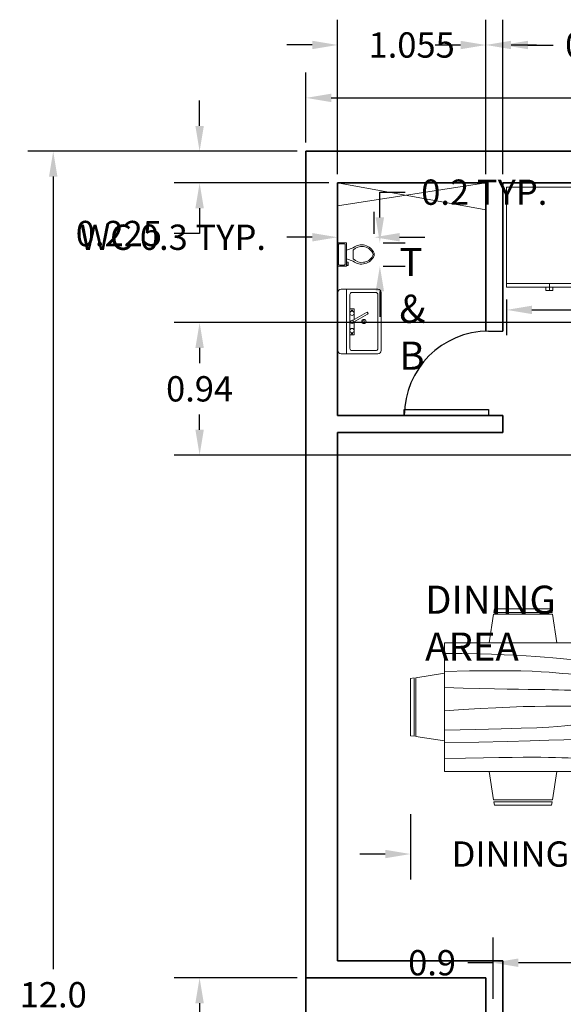
# Model space of a CAD drawing. Units: metres. Extents: x 4.8 to 18.3, y 28.2 to 89.8.
# Tile 2 of 4: x 4.8 to 8.6, y 36.6 to 43.6. Entities that reach past the tile are written whole.
import ezdxf

# ---------------------------------------------------------------- set-up
doc = ezdxf.new("R2010")
doc.units = ezdxf.units.M
doc.header["$MEASUREMENT"] = 0
doc.layers.get('Defpoints').update_dxf_attribs({"color": 3})
for name, color, linetype, lineweight in [('A-ANNO-DIMS', 2, 'Continuous', 18), ('A-AREA-IDEN', 7, 'Continuous', 25), ('A-DOOR', 3, 'Continuous', 25), ('A-EQPM', 8, 'Continuous', 18), ('A-FLOR-FIXT', 9, 'Continuous', 18), ('A-FURN', 8, 'Continuous', 18), ('A-WALL', 7, 'Continuous', 35)]:
    doc.layers.add(name, color=color, linetype=linetype, lineweight=lineweight)
doc.styles.get("Standard").update_dxf_attribs({"font": 'arial.ttf'})
doc.dimstyles.get("Standard").update_dxf_attribs({"dimtxt": 0.18, "dimasz": 0.18, "dimexe": 0.18, "dimexo": 0.0625, "dimgap": 0.09, "dimtad": 0, "dimtih": 1, "dimtoh": 1, "dimdec": 1, "dimzin": 0, "dimdsep": 46, "dimtxsty": 'Standard', "dimcen": 0.09, "dimadec": 0, "dimazin": 0, "dimtfac": 1, "dimtdec": 1, "dimtofl": 0, "dimtmove": 0, "dimatfit": 3, "dimfxl": 1, "dimtolj": 1, "dimtzin": 0, "dimarcsym": 0})

# ---------------------------------------------------------------- blocks, each defined once
blk = doc.blocks.new('*U3')
for p, q in [((0, 0), (0, -100)), ((600, 0), (600, -100))]:
    blk.add_line(p, q)
blk.add_lwpolyline([(0, 0), (0, 600), (43.75, 600), (43.75, 0)], close=True)
blk.add_arc((0, 0), 600, 0, 90)
blk = doc.blocks.new('Toilet - top')
for p, q in [((-10, -8.5), (-8, -8.5)), ((-10, -9.5), (-10, -8.5)), ((-8, -8.5), (-8, -8)), ((-7, -8), (-7, -9.5)), ((-4, -8), (-6, -14)), ((4, -8), (6, -14)), ((9.5, -6), (9.5, -2)), ((-7, -9.5), (-10, -9.5)), ((4, -14), (-4, -14))]:
    blk.add_line(p, q)
blk.add_lwpolyline([(10.5, -8), (10.5, 0), (-10.5, 0), (-10.5, -8)], close=True)
for points in [[(-9.5, -2), (-9.5, -6)], [(8.5, -1), (-8.5, -1)], [(-8.5, -7), (8.5, -7)]]:
    blk.add_lwpolyline(points)
for centre, radius, start, end in [((-8.62, -1.88), 0.884, 81.8699, 188.1301), ((-8.62, -6.12), 0.884, 171.8699, 278.1301), ((8.62, -1.88), 0.884, 351.8699, 98.1301), ((8.62, -6.12), 0.884, 261.8699, 8.1301), ((3.52, -21.58), 12.17, 141.46911, 247.97143), ((4.2, -21.82), 11.33, 136.36773, 238.94682), ((-3.52, -21.58), 12.17, 292.02843, 38.53071), ((-4.2, -21.82), 11.33, 301.05301, 43.63209), ((0, -27.88), 4, 245.73182, 294.26817), ((0, -29), 4, 254.86053, 285.13947)]:
    blk.add_arc(centre, radius, start, end)
blk = doc.blocks.new('Sink-single - 30 in top')
blk.add_line((-15, -3.999996), (15, -3.999996))
for points in [[(-13.5, 0), (13.5, 0)], [(-15, -18.499996), (-15, -1.5)], [(15, -1.5), (15, -18.499996)], [(-13.5, -17.499996), (-13.5, -6.499996)], [(-12.5, -5.499996), (12.5, -5.499996)], [(13.5, -6.499996), (13.5, -17.499996)], [(13.5, -19.999996), (-13.5, -19.999996)], [(12.5, -18.499996), (-12.5, -18.499996)]]:
    blk.add_lwpolyline(points)
for radius in [1, 0.5]:
    blk.add_circle((0, -11.999996), radius)
for centre, radius, start, end in [((-13.5, -1.5), 1.5, 90, 180), ((13.5, -1.5), 1.5, 0, 90), ((-12.5, -6.499996), 1, 90, 180), ((12.5, -6.499996), 1, 0, 90), ((-12.5, -17.499996), 1, 180, 270), ((12.5, -17.499996), 1, 270, 0), ((-13.5, -18.499996), 1.5, 180, 270), ((13.5, -18.499996), 1.5, 270, 0)]:
    blk.add_arc(centre, radius, start, end)
blk = doc.blocks.new('Faucet - kit sink top')
for p, q in [((-5.5, -0.75), (-5.5, -1.25)), ((-4.94278, -0.75), (-5.5, -0.75)), ((-5.5, -1.25), (-4.94278, -1.25)), ((-0.14775, -1.7441), (3.56698, -8.1782)), ((4.43301, -7.6782), (0.71828, -1.2441)), ((4.94278, -0.75), (5.5, -0.75)), ((5.5, -1.25), (4.94278, -1.25)), ((5.5, -0.75), (5.5, -1.25))]:
    blk.add_line(p, q)
blk.add_lwpolyline([(-0.00587, -2), (-6, -2), (-6, 0), (6, 0), (6, -2), (1.15195, -2)])
for centre, radius in [((-4, -1), 1), ((4, -1), 1), ((0, -1), 0.75)]:
    blk.add_circle(centre, radius)
blk.add_arc((4, -7.9282), 0.5, 210, 30)
blk = doc.blocks.new('Refrigerator-2 door - 36 in top')
for p, q in [((0, -26.999999), (36, -26.999999)), ((12, -26.999999), (12, -28.999999)), ((11, -27.999999), (11, -28.999999)), ((11, -28.999999), (13, -28.999999)), ((13, -28.999999), (13, -27.999999))]:
    blk.add_line(p, q)
blk.add_lwpolyline([(0, -27.999999), (0, 0), (36, 0), (36, -27.999999)], close=True)
blk = doc.blocks.new('Dining Set - 36 x 72 in.')
for p, q in [((-22.2343, 26.00059), (-23.4847, 17.99762)), ((-22.2304, 26), (-5.7608, 26)), ((-22, 27.5), (-22.1562, 26.50042)), ((-5.8416, 26.5), (-22.1534, 26.5)), ((-22, 27.5), (-6, 27.5)), ((-5.8437, 26.49966), (-6, 27.5)), ((-4.5152, 17.99762), (-5.7655, 25.99926)), ((5.7657, 26.00059), (4.5153, 17.99762)), ((5.7696, 26), (22.2392, 26)), ((6, 27.5), (5.8438, 26.50042)), ((22.1584, 26.5), (5.8466, 26.5)), ((6, 27.5), (22, 27.5)), ((22.1563, 26.49966), (22, 27.5)), ((23.4848, 17.99762), (22.2345, 25.99926)), ((36, 18), (-36, 18)), ((-36, 18), (-36, -18)), ((36, -18), (36, 18)), ((-44.0006, 8.23428), (-35.9976, 9.48474)), ((44.0006, 8.23428), (35.9976, 9.48474)), ((-45.5, 8), (-44.5004, 8.15617)), ((-45.5, 8), (-45.5, -8)), ((-44.5, -8.15843), (-44.5, 8.15338)), ((-44, 8.23041), (-44, -8.23915)), ((44, 8.23041), (44, -8.23915)), ((44.5, -8.15843), (44.5, 8.15338)), ((45.5, 8), (44.5005, 8.15617)), ((45.5, 8), (45.5, -8)), ((-44.4997, -8.15631), (-45.5, -8)), ((-35.9976, -9.48476), (-43.9993, -8.2345)), ((35.9976, -9.48476), (43.9993, -8.2345)), ((44.4997, -8.15631), (45.5, -8)), ((-36, -18), (36, -18)), ((-22.2343, -26.0006), (-23.4847, -17.99762)), ((-4.5152, -17.99762), (-5.7655, -25.99928)), ((5.7657, -26.0006), (4.5153, -17.99762)), ((23.4848, -17.99762), (22.2345, -25.99928)), ((-22.2304, -26), (-5.7608, -26)), ((-22, -27.5), (-22.1562, -26.50044)), ((-5.8416, -26.5), (-22.1534, -26.5)), ((-22, -27.5), (-6, -27.5)), ((-5.8437, -26.49967), (-6, -27.5)), ((5.7696, -26), (22.2392, -26)), ((6, -27.5), (5.8438, -26.50044)), ((22.1584, -26.5), (5.8466, -26.5)), ((6, -27.5), (22, -27.5)), ((22.1563, -26.49967), (22, -27.5))]:
    blk.add_line(p, q)
for points in [[(-36, 15), (-31.1772, 14.97754), (-26.8079, 14.91406), (-22.8538, 14.81543), (-19.276, 14.6875), (-16.0362, 14.53613), (-13.0957, 14.36718), (-10.4159, 14.18652), (-7.9583, 14), (-5.6904, 13.81315), (-3.6035, 13.63021), (-1.6954, 13.45508), (0.0365, 13.29166), (1.5945, 13.14388), (2.9811, 13.01562), (4.1988, 12.9108), (5.25, 12.83333), (6.1393, 12.78613), (6.8802, 12.76823), (7.4883, 12.77767), (7.9792, 12.8125), (8.3685, 12.87077), (8.6719, 12.95052), (8.9049, 13.0498), (9.0833, 13.16666), (9.2205, 13.29899), (9.3216, 13.44401), (9.3895, 13.59879), (9.4271, 13.76041), (9.4373, 13.92594), (9.4232, 14.09245), (9.3875, 14.257), (9.3333, 14.41666), (9.2638, 14.56917), (9.1836, 14.71484), (9.0975, 14.85465), (9.0104, 14.98958), (8.9272, 15.1206), (8.8529, 15.2487), (8.7922, 15.37483), (8.75, 15.5), (8.7305, 15.62467), (8.7344, 15.74739), (8.7617, 15.86621), (8.8125, 15.97916), (8.8867, 16.08431), (8.9844, 16.17968), (9.1055, 16.26334), (9.25, 16.33333), (9.4189, 16.38802), (9.6172, 16.42708), (9.8506, 16.45052), (10.125, 16.45833), (10.4463, 16.45052), (10.8203, 16.42708), (11.2529, 16.38802), (11.75, 16.33333), (12.3184, 16.26318), (12.9694, 16.17838), (13.7151, 16.07991), (14.5677, 15.96875), (15.5395, 15.84586), (16.6426, 15.71224), (17.8893, 15.56884), (19.2917, 15.41666), (20.859, 15.25667), (22.5879, 15.08984), (24.4721, 14.91715), (26.5052, 14.73958), (28.6809, 14.5581), (30.9929, 14.3737), (33.4347, 14.18733), (36, 14)], [(-36, 10), (-28.9766, 10.14274), (-23.1725, 10.20442), (-18.4241, 10.19775), (-14.5677, 10.13541), (-11.4399, 10.03011), (-8.877, 9.89453), (-6.7154, 9.74137), (-4.7917, 9.58333), (-2.9698, 9.43082), (-1.2246, 9.28515), (0.4415, 9.14534), (2.026, 9.01041), (3.5266, 8.87939), (4.9408, 8.7513), (6.266, 8.62516), (7.5, 8.5), (8.6411, 8.37549), (9.6914, 8.2539), (10.6538, 8.13818), (11.5312, 8.03125), (12.3267, 7.93603), (13.043, 7.85547), (13.6831, 7.79248), (14.25, 7.75), (14.7471, 7.7303), (15.1797, 7.73307), (15.5537, 7.75732), (15.875, 7.80208), (16.1494, 7.86637), (16.3828, 7.94922), (16.5811, 8.04964), (16.75, 8.16666), (16.8944, 8.29915), (17.0143, 8.44531), (17.1089, 8.60319), (17.1771, 8.77083), (17.218, 8.94629), (17.2305, 9.1276), (17.2137, 9.31282), (17.1667, 9.5), (17.0895, 9.6875), (16.987, 9.875), (16.8649, 10.0625), (16.7292, 10.25), (16.5856, 10.4375), (16.4401, 10.625), (16.2985, 10.8125), (16.1667, 11), (16.05, 11.18733), (15.9518, 11.3737), (15.8752, 11.5581), (15.8229, 11.73958), (15.798, 11.91715), (15.8034, 12.08984), (15.842, 12.25667), (15.9167, 12.41666), (16.0295, 12.56836), (16.1784, 12.70833), (16.3605, 12.83268), (16.5729, 12.9375), (16.8127, 13.01888), (17.0768, 13.07291), (17.3625, 13.0957), (17.6667, 13.08333), (17.9894, 13.03312), (18.3418, 12.94726), (18.7382, 12.82918), (19.1927, 12.68229), (19.7195, 12.51001), (20.3327, 12.31575), (21.0465, 12.10294), (21.875, 11.875), (22.8357, 11.63354), (23.959, 11.37304), (25.2786, 11.08618), (26.8282, 10.76562), (28.6414, 10.40405), (30.752, 9.99414), (33.1936, 9.52856), (36, 9)], [(-36, 5.5), (-30.7157, 5.3348), (-26.069, 5.20963), (-21.9946, 5.11767), (-18.4271, 5.05208), (-15.3009, 5.00602), (-12.5508, 4.97265), (-10.1112, 4.94515), (-7.9167, 4.91666), (-5.909, 4.88167), (-4.0586, 4.83984), (-2.3429, 4.79215), (-0.7396, 4.73958), (0.7739, 4.6831), (2.22, 4.6237), (3.6213, 4.56233), (5, 4.5), (6.373, 4.43782), (7.7344, 4.3776), (9.0723, 4.32129), (10.375, 4.27083), (11.6309, 4.22819), (12.8281, 4.19531), (13.9551, 4.17415), (15, 4.16666), (15.954, 4.17448), (16.819, 4.19791), (17.6001, 4.23698), (18.3021, 4.29166), (18.9299, 4.36198), (19.4883, 4.44791), (19.9823, 4.54948), (20.4167, 4.66666), (20.7969, 4.79899), (21.1302, 4.94401), (21.4245, 5.09879), (21.6875, 5.26041), (21.9271, 5.42594), (22.1511, 5.59245), (22.3672, 5.757), (22.5834, 5.91666), (22.8065, 6.06868), (23.0404, 6.21093), (23.2879, 6.34147), (23.5521, 6.45833), (23.8358, 6.55957), (24.142, 6.64323), (24.4735, 6.70735), (24.8334, 6.75), (25.2235, 6.76969), (25.642, 6.76692), (26.0858, 6.74267), (26.5521, 6.69791), (27.0379, 6.63362), (27.5404, 6.55078), (28.0565, 6.45036), (28.5834, 6.33333), (29.1242, 6.19987), (29.7071, 6.04687), (30.3661, 5.87044), (31.1354, 5.66666), (32.0493, 5.43164), (33.142, 5.16146), (34.4475, 4.85221), (36, 4.5)], [(-36, -1), (-30.7915, -0.6591), (-26.0195, -0.38216), (-21.6519, -0.16284), (-17.6563, 0.00521), (-14.0005, 0.12833), (-10.6523, 0.21289), (-7.5796, 0.26522), (-4.75, 0.29166), (-2.134, 0.29793), (0.2878, 0.28711), (2.5317, 0.26163), (4.6146, 0.22396), (6.5529, 0.17651), (8.3633, 0.12174), (10.0623, 0.06209), (11.6667, 0), (13.1899, -0.06201), (14.6341, -0.1211), (15.9982, -0.17432), (17.2813, -0.21875), (18.4823, -0.25147), (19.6003, -0.26953), (20.6343, -0.27002), (21.5834, -0.25), (22.4481, -0.20768), (23.2357, -0.14584), (23.9549, -0.06836), (24.6146, 0.02083), (25.2235, 0.11784), (25.7904, 0.21875), (26.3241, 0.31966), (26.8334, 0.41666), (27.3265, 0.50618), (27.8099, 0.58593), (28.2894, 0.65397), (28.7709, 0.70833), (29.2601, 0.74707), (29.763, 0.76823), (30.2855, 0.76985), (30.8334, 0.75), (31.4088, 0.70784), (31.9994, 0.64713), (32.589, 0.57275), (33.1615, 0.48958), (33.7008, 0.4025), (34.1908, 0.3164), (34.6153, 0.23616), (34.9584, 0.16666), (35.2099, 0.11165), (35.3848, 0.07031), (35.504, 0.04069), (35.5886, 0.02083), (35.6594, 0.00879), (35.7377, 0.0026), (35.8442, 0.00032), (36, 0)], [(-36, -6.5), (-27.1843, -6.31267), (-20.084, -6.1263), (-14.469, -5.9419), (-10.1094, -5.76042), (-6.7752, -5.58285), (-4.2363, -5.41016), (-2.2629, -5.24333), (-0.625, -5.08334), (0.8708, -4.93099), (2.2715, -4.78646), (3.5872, -4.64974), (4.8281, -4.52084), (6.0046, -4.39974), (7.127, -4.28646), (8.2053, -4.18099), (9.25, -4.08334), (10.2705, -3.99382), (11.2734, -3.91407), (12.2647, -3.84603), (13.25, -3.79167), (14.2354, -3.75293), (15.2266, -3.73177), (16.2295, -3.73015), (17.25, -3.75), (18.2912, -3.79248), (19.3451, -3.85547), (20.4009, -3.93604), (21.4479, -4.03125), (22.4754, -4.13819), (23.4727, -4.25391), (24.4289, -4.37549), (25.3334, -4.5), (26.1785, -4.62492), (26.9694, -4.74935), (27.7145, -4.87281), (28.4219, -4.99479), (29.1, -5.11483), (29.7572, -5.23242), (30.4016, -5.34709), (31.0417, -5.45834), (31.6837, -5.56437), (32.3262, -5.65821), (32.9658, -5.73153), (33.599, -5.77604), (34.2224, -5.78345), (34.8327, -5.74545), (35.4264, -5.65373), (36, -5.5)], [(-36, -10), (-26.4022, -9.81299), (-18.4675, -9.62891), (-11.9839, -9.45069), (-6.7396, -9.28125), (-2.5226, -9.12354), (0.8789, -8.98047), (3.6769, -8.85498), (6.0833, -8.75), (8.2767, -8.66765), (10.3021, -8.60677), (12.1712, -8.56543), (13.8958, -8.54167), (15.4876, -8.53353), (16.9583, -8.53907), (18.3197, -8.55632), (19.5834, -8.58334), (20.7616, -8.61841), (21.8685, -8.66081), (22.9188, -8.71004), (23.9271, -8.76563), (24.9081, -8.82707), (25.8763, -8.89388), (26.8465, -8.96558), (27.8334, -9.04167), (28.8474, -9.12118), (29.8828, -9.20117), (30.93, -9.27824), (31.9792, -9.34896), (33.0205, -9.40991), (34.0443, -9.45768), (35.0407, -9.48885), (36, -9.5)], [(-36, -14.5), (-30.0881, -14.33513), (-25.0332, -14.21224), (-20.7312, -14.12647), (-17.0781, -14.07292), (-13.97, -14.04671), (-11.3027, -14.04297), (-8.9724, -14.05681), (-6.875, -14.08334), (-4.9224, -14.11833), (-3.0905, -14.16016), (-1.3709, -14.20785), (0.2448, -14.26042), (1.7647, -14.3169), (3.1973, -14.3763), (4.5507, -14.43767), (5.8333, -14.5), (7.0554, -14.5621), (8.235, -14.62175), (9.3922, -14.67652), (10.5469, -14.72396), (11.7192, -14.76164), (12.929, -14.78711), (14.1965, -14.79794), (15.5417, -14.79167), (16.9933, -14.76424), (18.6152, -14.70508), (20.4804, -14.60197), (22.6615, -14.44271), (25.2312, -14.21509), (28.2624, -13.9069), (31.8277, -13.50594), (36, -13)]]:
    blk.add_lwpolyline(points)
blk = doc.blocks.new('*D18')
at = {"layer": 'A-ANNO-DIMS', "color": 0, "lineweight": -2, "transparency": 16777216}
for p, q in [((6.731, 42.6633), (4.8163, 42.6633)), ((4.9963, 42.4833), (4.9963, 36.8452)), ((4.9963, 30.8433), (4.9963, 36.4813)), ((6.731, 30.6633), (4.8163, 30.6633))]:
    blk.add_line(p, q, dxfattribs=at)
at = {"layer": 'A-ANNO-DIMS', "color": 0, "transparency": 16777216}
for points in [[(4.9663, 42.4833), (5.0263, 42.4833), (4.9963, 42.6633)], [(4.9663, 30.8433), (5.0263, 30.8433), (4.9963, 30.6633)]]:
    blk.add_solid(points, dxfattribs=at)
at = {"layer": 'Defpoints', "color": 0, "transparency": 16777216}
for p in [(6.7935, 42.6633), (4.9963, 30.6633), (6.7935, 30.6633)]:
    blk.add_point(p, dxfattribs=at)
at = {"layer": 'A-ANNO-DIMS', "color": 0, "transparency": 16777216, "insert": (4.9963, 36.6633), "char_height": 0.18, "attachment_point": 5}
blk.add_mtext('\\A1;12.0', dxfattribs=at)
blk = doc.blocks.new('*D22')
at = {"layer": 'A-ANNO-DIMS', "color": 0, "lineweight": -2, "transparency": 16777216}
for p, q in [((6.7935, 42.7258), (6.7935, 43.223)), ((12.2935, 42.7258), (12.2935, 43.223)), ((6.9735, 43.043), (9.289, 43.043)), ((12.1135, 43.043), (9.798, 43.043))]:
    blk.add_line(p, q, dxfattribs=at)
at = {"layer": 'A-ANNO-DIMS', "color": 0, "transparency": 16777216}
for points in [[(6.9735, 43.073), (6.9735, 43.013), (6.7935, 43.043)], [(12.1135, 43.073), (12.1135, 43.013), (12.2935, 43.043)]]:
    blk.add_solid(points, dxfattribs=at)
at = {"layer": 'Defpoints', "color": 0, "transparency": 16777216}
for p in [(12.2935, 43.043), (6.7935, 42.6633), (12.2935, 42.6633)]:
    blk.add_point(p, dxfattribs=at)
at = {"layer": 'A-ANNO-DIMS', "color": 0, "transparency": 16777216, "insert": (9.5435, 43.043), "char_height": 0.18, "attachment_point": 5}
blk.add_mtext('\\A1;5.5', dxfattribs=at)
blk = doc.blocks.new('*D32')
at = {"layer": 'A-ANNO-DIMS', "color": 0, "lineweight": -2, "transparency": 16777216}
for p, q in [((7.0185, 42.0749), (7.0185, 42.2317)), ((7.2803, 42.0749), (7.2803, 42.2317)), ((6.8385, 42.0517), (6.6585, 42.0517)), ((7.4603, 42.0517), (7.6403, 42.0517))]:
    blk.add_line(p, q, dxfattribs=at)
at = {"layer": 'A-ANNO-DIMS', "color": 0, "transparency": 16777216}
for points in [[(6.8385, 42.0817), (6.8385, 42.0217), (7.0185, 42.0517)], [(7.4603, 42.0817), (7.4603, 42.0217), (7.2803, 42.0517)]]:
    blk.add_solid(points, dxfattribs=at)
at = {"layer": 'Defpoints', "color": 0, "transparency": 16777216}
for p in [(7.0185, 42.0517), (7.0185, 42.0124), (7.2803, 42.0124)]:
    blk.add_point(p, dxfattribs=at)
at = {"layer": 'A-ANNO-DIMS', "color": 0, "transparency": 16777216, "insert": (5.8474, 42.0517), "char_height": 0.18, "attachment_point": 5}
blk.add_mtext('\\A1;WC 0.3 TYP.', dxfattribs=at)
blk = doc.blocks.new('*D33')
at = {"layer": 'A-ANNO-DIMS', "color": 0, "lineweight": -2, "transparency": 16777216}
for p, q in [((7.3196, 42.1924), (7.3196, 42.3724)), ((7.3196, 42.3724), (7.4996, 42.3724)), ((7.3428, 42.0124), (7.4996, 42.0124)), ((7.3428, 41.846), (7.4996, 41.846)), ((7.3196, 41.666), (7.3196, 41.486))]:
    blk.add_line(p, q, dxfattribs=at)
at = {"layer": 'A-ANNO-DIMS', "color": 0, "transparency": 16777216}
for points in [[(7.2896, 42.1924), (7.3496, 42.1924), (7.3196, 42.0124)], [(7.2896, 41.666), (7.3496, 41.666), (7.3196, 41.846)]]:
    blk.add_solid(points, dxfattribs=at)
at = {"layer": 'Defpoints', "color": 0, "transparency": 16777216}
for p in [(7.2803, 42.0124), (7.3196, 42.0124), (7.2803, 41.846)]:
    blk.add_point(p, dxfattribs=at)
at = {"layer": 'A-ANNO-DIMS', "color": 0, "transparency": 16777216, "insert": (8.0626, 42.3724), "char_height": 0.18, "attachment_point": 5}
blk.add_mtext('\\A1;0.2 TYP.', dxfattribs=at)
blk = doc.blocks.new('*D36')
at = {"layer": 'A-ANNO-DIMS', "color": 0, "lineweight": -2, "transparency": 16777216}
for p, q in [((8.2211, 41.6097), (8.2211, 41.355)), ((9.1355, 41.6097), (9.1355, 41.355)), ((8.4011, 41.535), (8.9555, 41.535)), ((9.1355, 41.535), (9.3155, 41.535))]:
    blk.add_line(p, q, dxfattribs=at)
at = {"layer": 'A-ANNO-DIMS', "color": 0, "transparency": 16777216}
for points in [[(8.4011, 41.565), (8.4011, 41.505), (8.2211, 41.535)], [(8.9555, 41.565), (8.9555, 41.505), (9.1355, 41.535)]]:
    blk.add_solid(points, dxfattribs=at)
at = {"layer": 'Defpoints', "color": 0, "transparency": 16777216}
for p in [(8.2211, 41.6722), (9.1355, 41.6722), (9.1355, 41.535)]:
    blk.add_point(p, dxfattribs=at)
at = {"layer": 'A-ANNO-DIMS', "color": 0, "transparency": 16777216, "insert": (10.5987, 41.535), "char_height": 0.18, "attachment_point": 5}
blk.add_mtext('\\A1;REFRIGERATOR 0.9', dxfattribs=at)
blk = doc.blocks.new('*D41')
at = {"layer": 'A-ANNO-DIMS', "color": 0, "lineweight": -2, "transparency": 16777216}
for p, q in [((8.1252, 36.6335), (8.1252, 37.071)), ((9.0565, 36.6335), (9.0565, 37.071)), ((8.1252, 36.891), (7.9452, 36.891)), ((8.8765, 36.891), (8.3052, 36.891))]:
    blk.add_line(p, q, dxfattribs=at)
at = {"layer": 'A-ANNO-DIMS', "color": 0, "transparency": 16777216}
for points in [[(8.3052, 36.921), (8.3052, 36.861), (8.1252, 36.891)], [(8.8765, 36.921), (8.8765, 36.861), (9.0565, 36.891)]]:
    blk.add_solid(points, dxfattribs=at)
at = {"layer": 'Defpoints', "color": 0, "transparency": 16777216}
for p in [(8.1252, 36.891), (8.1252, 36.571), (9.0565, 36.571)]:
    blk.add_point(p, dxfattribs=at)
at = {"layer": 'A-ANNO-DIMS', "color": 0, "transparency": 16777216, "insert": (7.6911, 36.891), "char_height": 0.18, "attachment_point": 5}
blk.add_mtext('\\A1;0.9', dxfattribs=at)
blk = doc.blocks.new('*D44')
at = {"layer": 'A-ANNO-DIMS', "color": 0, "lineweight": -2, "transparency": 16777216}
for p, q in [((7.5379, 37.9483), (7.5379, 37.4841)), ((9.8493, 37.9483), (9.8493, 37.4841)), ((7.3579, 37.6641), (7.1779, 37.6641)), ((10.0293, 37.6641), (10.2093, 37.6641))]:
    blk.add_line(p, q, dxfattribs=at)
at = {"layer": 'A-ANNO-DIMS', "color": 0, "transparency": 16777216}
for points in [[(7.3579, 37.6941), (7.3579, 37.6341), (7.5379, 37.6641)], [(10.0293, 37.6941), (10.0293, 37.6341), (9.8493, 37.6641)]]:
    blk.add_solid(points, dxfattribs=at)
at = {"layer": 'Defpoints', "color": 0, "transparency": 16777216}
for p in [(7.5379, 38.0108), (9.8493, 38.0108), (9.8493, 37.6641)]:
    blk.add_point(p, dxfattribs=at)
at = {"layer": 'A-ANNO-DIMS', "color": 0, "transparency": 16777216, "insert": (8.6936, 37.6641), "char_height": 0.18, "attachment_point": 5}
blk.add_mtext('\\A1;DINING SET 2.3', dxfattribs=at)
blk = doc.blocks.new('*D47')
at = {"layer": 'A-ANNO-DIMS', "color": 0, "lineweight": -2, "transparency": 16777216}
for p, q in [((6.731, 36.7833), (5.8575, 36.7833)), ((6.0375, 36.6033), (6.0375, 33.9052)), ((6.0375, 30.8433), (6.0375, 33.5413)), ((6.731, 30.6633), (5.8575, 30.6633))]:
    blk.add_line(p, q, dxfattribs=at)
at = {"layer": 'A-ANNO-DIMS', "color": 0, "transparency": 16777216}
for points in [[(6.0075, 36.6033), (6.0675, 36.6033), (6.0375, 36.7833)], [(6.0075, 30.8433), (6.0675, 30.8433), (6.0375, 30.6633)]]:
    blk.add_solid(points, dxfattribs=at)
at = {"layer": 'Defpoints', "color": 0, "transparency": 16777216}
for p in [(6.0375, 36.7833), (6.7935, 36.7833), (6.7935, 30.6633)]:
    blk.add_point(p, dxfattribs=at)
at = {"layer": 'A-ANNO-DIMS', "color": 0, "transparency": 16777216, "insert": (6.0375, 33.7233), "char_height": 0.18, "attachment_point": 5}
blk.add_mtext('\\A1;6.12', dxfattribs=at)
blk = doc.blocks.new('*D54')
at = {"layer": 'A-ANNO-DIMS', "color": 0, "lineweight": -2, "transparency": 16777216}
for p, q in [((7.018483, 42.50075), (7.018483, 43.59925)), ((8.073483, 42.50075), (8.073483, 43.59925)), ((6.838483, 43.41925), (6.658483, 43.41925)), ((8.253483, 43.41925), (8.433483, 43.41925))]:
    blk.add_line(p, q, dxfattribs=at)
at = {"layer": 'A-ANNO-DIMS', "color": 0, "transparency": 16777216}
for points in [[(6.838483, 43.44925), (6.838483, 43.38925), (7.018483, 43.41925)], [(8.253483, 43.44925), (8.253483, 43.38925), (8.073483, 43.41925)]]:
    blk.add_solid(points, dxfattribs=at)
at = {"layer": 'Defpoints', "color": 0, "transparency": 16777216}
for p in [(8.073483, 43.41925), (7.018483, 42.43825), (8.073483, 42.43825)]:
    blk.add_point(p, dxfattribs=at)
at = {"layer": 'A-ANNO-DIMS', "color": 0, "transparency": 16777216, "insert": (7.545983, 43.41925), "char_height": 0.18, "attachment_point": 5}
blk.add_mtext('\\A1;1.055', dxfattribs=at)
blk = doc.blocks.new('*D59')
at = {"layer": 'A-ANNO-DIMS', "color": 0, "lineweight": -2, "transparency": 16777216}
for p, q in [((8.9037, 41.4446), (5.8575, 41.4446)), ((6.0375, 41.2646), (6.0375, 41.1553)), ((6.0375, 40.6822), (6.0375, 40.7915)), ((8.9037, 40.5022), (5.8575, 40.5022))]:
    blk.add_line(p, q, dxfattribs=at)
at = {"layer": 'A-ANNO-DIMS', "color": 0, "transparency": 16777216}
for points in [[(6.0075, 41.2646), (6.0675, 41.2646), (6.0375, 41.4446)], [(6.0075, 40.6822), (6.0675, 40.6822), (6.0375, 40.5022)]]:
    blk.add_solid(points, dxfattribs=at)
at = {"layer": 'Defpoints', "color": 0, "transparency": 16777216}
for p in [(6.0375, 41.4446), (8.9662, 41.4446), (8.9662, 40.5022)]:
    blk.add_point(p, dxfattribs=at)
at = {"layer": 'A-ANNO-DIMS', "color": 0, "transparency": 16777216, "insert": (6.0375, 40.9734), "char_height": 0.18, "attachment_point": 5}
blk.add_mtext('\\A1;0.94', dxfattribs=at)
blk = doc.blocks.new('*D62')
at = {"layer": 'A-ANNO-DIMS', "color": 0, "lineweight": -2, "transparency": 16777216}
for p, q in [((6.0375, 42.8433), (6.0375, 43.0233)), ((6.731, 42.6633), (5.8575, 42.6633)), ((6.956, 42.4383), (5.8575, 42.4383)), ((6.0375, 42.2583), (6.0375, 42.0782)), ((6.0375, 42.0782), (5.8575, 42.0782))]:
    blk.add_line(p, q, dxfattribs=at)
at = {"layer": 'A-ANNO-DIMS', "color": 0, "transparency": 16777216}
for points in [[(6.0075, 42.8433), (6.0675, 42.8433), (6.0375, 42.6633)], [(6.0075, 42.2583), (6.0675, 42.2583), (6.0375, 42.4383)]]:
    blk.add_solid(points, dxfattribs=at)
at = {"layer": 'Defpoints', "color": 0, "transparency": 16777216}
for p in [(6.7935, 42.6633), (6.0375, 42.4383), (7.0185, 42.4383)]:
    blk.add_point(p, dxfattribs=at)
at = {"layer": 'A-ANNO-DIMS', "color": 0, "transparency": 16777216, "insert": (5.4631, 42.0782), "char_height": 0.18, "attachment_point": 5}
blk.add_mtext('\\A1;0.225', dxfattribs=at)
blk = doc.blocks.new('*D63')
at = {"layer": 'A-ANNO-DIMS', "color": 0, "lineweight": -2, "transparency": 16777216}
for p, q in [((8.0735, 42.5007), (8.0735, 43.5992)), ((8.1935, 42.5007), (8.1935, 43.5992)), ((7.8935, 43.4192), (7.7135, 43.4192)), ((8.3735, 43.4192), (8.5535, 43.4192))]:
    blk.add_line(p, q, dxfattribs=at)
at = {"layer": 'A-ANNO-DIMS', "color": 0, "transparency": 16777216}
for points in [[(7.8935, 43.4492), (7.8935, 43.3892), (8.0735, 43.4192)], [(8.3735, 43.4492), (8.3735, 43.3892), (8.1935, 43.4192)]]:
    blk.add_solid(points, dxfattribs=at)
at = {"layer": 'Defpoints', "color": 0, "transparency": 16777216}
for p in [(8.1935, 43.4192), (8.0735, 42.4382), (8.1935, 42.4382)]:
    blk.add_point(p, dxfattribs=at)
at = {"layer": 'A-ANNO-DIMS', "color": 0, "transparency": 16777216, "insert": (8.8763, 43.4192), "char_height": 0.18, "attachment_point": 5}
blk.add_mtext('\\A1;0.12', dxfattribs=at)

msp = doc.modelspace()

# ---------------------------------------------------------------- linework, layer by layer
at = {"layer": 'A-FLOR-FIXT'}
for p, q in [((7.0185, 42.2763), (8.0735, 42.4382)), ((7.0185, 42.4382), (8.0735, 42.2464))]:
    msp.add_line(p, q, dxfattribs=at)
at = {"layer": 'A-WALL'}
for p, q in [((6.7935, 42.6632), (14.7935, 42.6632)), ((6.7935, 30.6633), (6.7935, 42.6632)), ((7.0185, 42.4382), (8.0735, 42.4382)), ((7.0185, 40.7833), (7.0185, 42.4382)), ((8.0735, 41.3829), (8.0735, 42.4382)), ((8.1935, 42.4382), (12.1735, 42.4382)), ((8.1935, 41.3833), (8.1935, 42.4382)), ((7.0185, 40.7833), (8.1935, 40.7833)), ((8.1935, 40.6633), (8.1935, 40.7833)), ((7.0185, 40.6633), (8.1935, 40.6633)), ((7.0185, 36.9033), (7.0185, 40.6633)), ((7.0185, 36.9033), (8.1935, 36.9033)), ((8.1935, 33.4333), (8.1935, 36.9033)), ((6.7935, 36.7833), (8.0735, 36.7833)), ((8.0735, 30.6633), (8.0735, 36.7833))]:
    msp.add_line(p, q, dxfattribs=at)

# ---------------------------------------------------------------- block references
at = {"layer": 'A-DOOR', "xscale": 0.001, "yscale": 0.001, "zscale": 0.001, "rotation": 90}
msp.add_blockref('*U3', (8.0935, 40.7833), dxfattribs=at)
at = {"layer": 'A-EQPM', "xscale": 0.0254, "yscale": 0.0254, "zscale": 0.0254}
msp.add_blockref('Refrigerator-2 door - 36 in top', (8.2211, 42.4088), dxfattribs=at)
at = {"layer": 'A-FLOR-FIXT', "rotation": 90}
for name, p, xscale, yscale, zscale in [('Toilet - top', (7.0185, 41.9292), 0.0079224064411582, 0.0079224064411582, 0.0079224064411582), ('Sink-single - 30 in top', (7.0218, 41.4523), 0.0153508848932381, 0.0153508848932381, 0.0153508848932381), ('Faucet - kit sink top', (7.1063, 41.4492), 0.0153508848932381, 0.0153508848932381, 0.0153508848932381)]:
    msp.add_blockref(name, p, dxfattribs=dict(at, xscale=xscale, yscale=yscale, zscale=zscale))
at = {"layer": 'A-FURN', "xscale": 0.0254, "yscale": 0.0254, "zscale": 0.0254}
msp.add_blockref('Dining Set - 36 x 72 in.', (8.6936, 38.7093), dxfattribs=at)

# ---------------------------------------------------------------- texts
at = {"layer": 'A-AREA-IDEN', "char_height": 0.2, "attachment_point": 1}
for s, width, insert in [('T & B', 0.334444, (7.4587, 41.9763)), ('DINING AREA', 0.829678, (7.642, 39.5734))]:
    msp.add_mtext_dynamic_manual_height_columns(s, width=width, gutter_width=1, heights=[0], dxfattribs=dict(at, insert=insert))

# ---------------------------------------------------------------- dimensions: what is measured, and where the dimension line sits
at = {"layer": 'A-ANNO-DIMS'}
for base, p1, p2, override, picture, middle in [((8.0735, 43.4192), (7.0185, 42.4382), (8.0735, 42.4382), {"dimdec": 3, "dimlfac": 1, "dimrnd": 0, "dimzin": 0, "dimdsep": 46, "dimlunit": 2}, '*D54', (7.546, 43.4192)), ((8.1935, 43.4192), (8.0735, 42.4382), (8.1935, 42.4382), {"dimdec": 2, "dimlfac": 1, "dimrnd": 0, "dimzin": 0, "dimdsep": 46, "dimlunit": 2}, '*D63', (8.8763, 43.4192)), ((12.2935, 43.043), (6.7935, 42.6632), (12.2935, 42.6632), {"dimclrd": 0, "dimclre": 0, "dimclrt": 0}, '*D22', (9.5435, 43.043))]:
    dim = msp.add_linear_dim(base=base, p1=p1, p2=p2, dimstyle='Standard', override=override, dxfattribs=at)
    dim.commit()
    dim.dimension.update_dxf_attribs({"geometry": picture, "text_midpoint": middle})
for base, p1, p2, angle, override, picture, middle in [((6.0375, 42.4382), (6.7935, 42.6632), (7.0185, 42.4382), 90, {"dimdec": 3, "dimlfac": 1, "dimrnd": 0, "dimzin": 0, "dimdsep": 46, "dimlunit": 2}, '*D62', (5.4631, 42.0782)), ((4.9963, 30.6633), (6.7935, 42.6632), (6.7935, 30.6633), 90, {"dimclrd": 0, "dimclre": 0, "dimclrt": 0}, '*D18', (4.9963, 36.6633)), ((6.0375, 41.4446), (8.9662, 40.5022), (8.9662, 41.4446), 90, {"dimdec": 2, "dimlfac": 1, "dimrnd": 0, "dimzin": 0, "dimdsep": 46, "dimlunit": 2}, '*D59', (6.0375, 40.9734)), ((8.1252, 36.891), (9.0565, 36.571), (8.1252, 36.571), 180, {"dimdec": 1, "dimlfac": 1, "dimrnd": 0, "dimzin": 0, "dimdsep": 46, "dimlunit": 2}, '*D41', (7.6911, 36.891)), ((6.0375, 36.7833), (6.7935, 30.6633), (6.7935, 36.7833), 90, {"dimdec": 2, "dimlfac": 1, "dimrnd": 0, "dimzin": 0, "dimdsep": 46, "dimlunit": 2}, '*D47', (6.0375, 33.7233))]:
    dim = msp.add_linear_dim(base=base, p1=p1, p2=p2, angle=angle, dimstyle='Standard', override=override, dxfattribs=at)
    dim.commit()
    dim.dimension.update_dxf_attribs({"geometry": picture, "text_midpoint": middle})
for base, p1, p2, angle, text, picture, middle in [((7.3196, 42.0124), (7.2803, 41.846), (7.2803, 42.0124), 90, '<> TYP.', '*D33', (8.0626, 42.3724)), ((7.0185, 42.0517), (7.2803, 42.0124), (7.0185, 42.0124), 180, 'WC <> TYP.', '*D32', (5.8474, 42.0517))]:
    dim = msp.add_linear_dim(base=base, p1=p1, p2=p2, angle=angle, text=text, dimstyle='Standard', override={"dimdec": 1, "dimlfac": 1, "dimrnd": 0, "dimzin": 0, "dimdsep": 46, "dimlunit": 2}, dxfattribs=at)
    dim.commit()
    dim.dimension.update_dxf_attribs({"geometry": picture, "text_midpoint": middle})
for base, p1, p2, text, picture, middle in [((9.1355, 41.535), (8.2211, 41.6722), (9.1355, 41.6722), 'REFRIGERATOR <>', '*D36', (10.5987, 41.535)), ((9.8493, 37.6641), (7.5379, 38.0108), (9.8493, 38.0108), 'DINING SET <>', '*D44', (8.6936, 37.6641))]:
    dim = msp.add_linear_dim(base=base, p1=p1, p2=p2, text=text, dimstyle='Standard', override={"dimdec": 1, "dimlfac": 1, "dimrnd": 0, "dimzin": 0, "dimdsep": 46, "dimlunit": 2}, dxfattribs=at)
    dim.commit()
    dim.dimension.update_dxf_attribs({"geometry": picture, "text_midpoint": middle})

doc.saveas('drawing.dxf')
